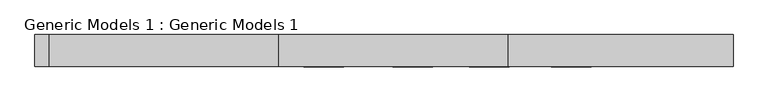
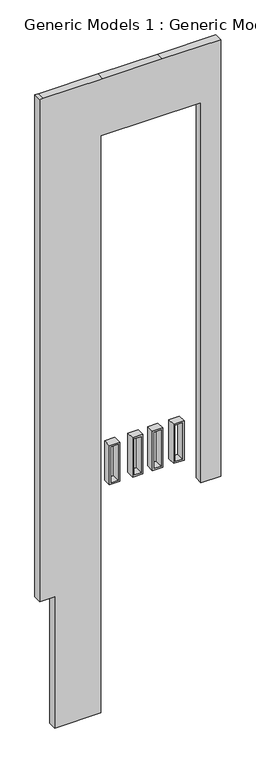
"""IFC4 building model written with IfcOpenShell, lengths in millimetres: proxy geometry, Generic Models 1 : Generic Models 1."""

from ifc_helpers import new_model, si_unit, frame, origin, place, context, project, spatial, polyline, outline, extrude, source, transform, mapped, element, save


def generic_models_1_generic_models_1_d955dbe1(model_context):
    return source(origin(), model_context, "Body", "SweptSolid", [
        extrude(outline(polyline([(9981.2110614, -13864.7667709), (9981.2110614, -13921.9167709), (1828.8, -13921.9167709), (1828.8, -13693.3167709), (-304.8, -13693.3167709), (-304.8, -12982.1167709), (9066.8256285, -12982.1167709), (9066.8256285, -11445.4167709), (2895.6, -11445.4167709), (2895.6, -11140.6167709), (9981.2110614, -11140.6167709), (9981.2110614, -12035.9667709), (9981.2110614, -12950.3667709), (9981.2110614, -13864.7667709)])), frame((0.0, -4345.3637867, 0.0), z_axis=(0.0, 1.0, 0.0), x_axis=(0.0, 0.0, 1.0)), (0.0, 0.0, 1.0), 127.0),
        extrude(outline(polyline([(3989.5004539, -12692.2660532), (3989.5004539, -12851.4762568), (3352.8, -12851.4762568), (3352.8, -12692.2660532), (3989.5004539, -12692.2660532)]), holes=[polyline([(3964.1004539, -12717.6660532), (3378.2, -12717.6660532), (3378.2, -12826.0762568), (3964.1004539, -12826.0762568), (3964.1004539, -12717.6660532)])]), frame((0.0, -4345.3637867, 0.0), z_axis=(0.0, 1.0, 0.0), x_axis=(0.0, 0.0, 1.0)), (0.0, 0.0, 1.0), 127.0),
        extrude(outline(polyline([(3352.8, -12495.8762568), (3352.8, -12336.6660532), (3989.5004539, -12336.6660532), (3989.5004539, -12495.8762568), (3352.8, -12495.8762568)]), holes=[polyline([(3378.2, -12470.4762568), (3964.1004539, -12470.4762568), (3964.1004539, -12362.0660532), (3378.2, -12362.0660532), (3378.2, -12470.4762568)])]), frame((0.0, -4345.3637867, 0.0), z_axis=(0.0, 1.0, 0.0), x_axis=(0.0, 0.0, 1.0)), (0.0, 0.0, 1.0), 127.0),
        extrude(outline(polyline([(3352.8, -12191.0762568), (3352.8, -12031.8660532), (3989.5004539, -12031.8660532), (3989.5004539, -12191.0762568), (3352.8, -12191.0762568)]), holes=[polyline([(3378.2, -12165.6762568), (3964.1004539, -12165.6762568), (3964.1004539, -12057.2660532), (3378.2, -12057.2660532), (3378.2, -12165.6762568)])]), frame((0.0, -4345.3637867, 0.0), z_axis=(0.0, 1.0, 0.0), x_axis=(0.0, 0.0, 1.0)), (0.0, 0.0, 1.0), 127.0),
        extrude(outline(polyline([(3352.8, -11864.5167709), (3352.8, -11705.3065673), (3989.5004539, -11705.3065673), (3989.5004539, -11864.5167709), (3352.8, -11864.5167709)]), holes=[polyline([(3378.2, -11839.1167709), (3964.1004539, -11839.1167709), (3964.1004539, -11730.7065673), (3378.2, -11730.7065673), (3378.2, -11839.1167709)])]), frame((0.0, -4345.3637867, 0.0), z_axis=(0.0, 1.0, 0.0), x_axis=(0.0, 0.0, 1.0)), (0.0, 0.0, 1.0), 127.0),
    ])


if __name__ == "__main__":
    model = new_model("IFC4")
    model_context = context("Model", 3, world=origin())
    ifc_project = project(units=[si_unit("LENGTHUNIT", "METRE", prefix="MILLI")], contexts=[model_context])
    site = spatial("IfcSite", under=ifc_project)
    building = spatial("IfcBuilding", under=site)
    placement = place(None, origin())
    generic_models_1_generic_models_1_shape = generic_models_1_generic_models_1_d955dbe1(model_context)
    element("IfcBuildingElementProxy", 1, Name="Generic Models 1 : Generic Models 1", ObjectType="Generic Models 1 : Generic Models 1", at=placement, inside=building, context=model_context, shape_type="MappedRepresentation", body=[
        mapped(generic_models_1_generic_models_1_shape, transform((0.0, 0.0, 0.0), x_axis=(1.0, 0.0, 0.0), y_axis=(0.0, 1.0, 0.0), z_axis=(0.0, 0.0, 1.0))),
    ])
    save(model, "model.ifc")
